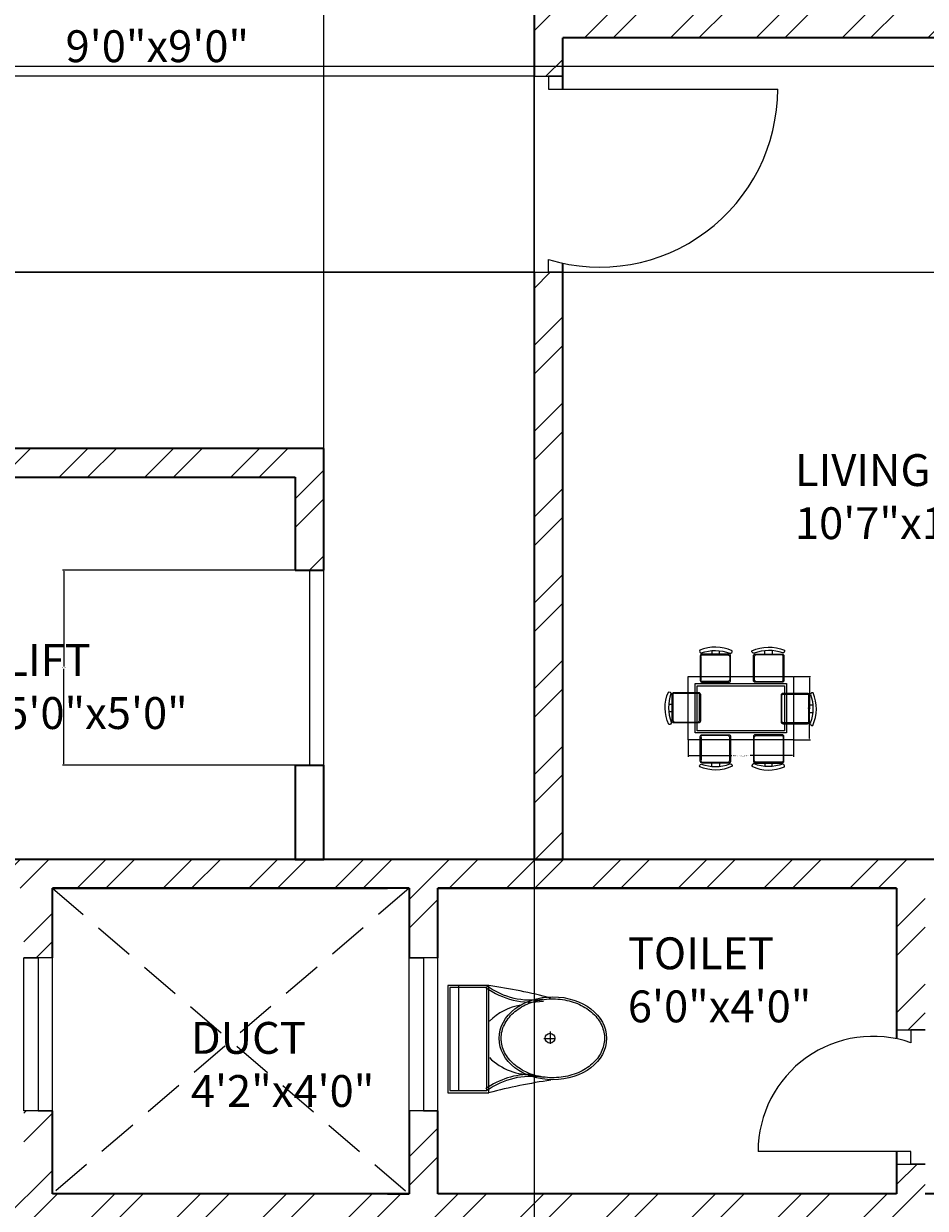
# Model space of a CAD drawing. Units: inches. Extents: x 1570 to 2186, y 1575 to 2421.
# Tile 4 of 10: x 1833 to 1975, y 1859 to 2045. Entities that reach past the tile are written whole.
import ezdxf

# ---------------------------------------------------------------- set-up
doc = ezdxf.new("R2010")
doc.units = ezdxf.units.IN
doc.linetypes.add('DASHED2', pattern=[9.525, 6.35, -3.175])
for name, color, linetype, lineweight in [('A-ANNO-DIMS', 2, 'Continuous', 18), ('A-AREA-IDEN', 7, 'Continuous', 18), ('A-DOOR', 201, 'Continuous', 18), ('A-FLOR-FIXT', 9, 'Continuous', 18), ('A-FLOR-OPEN', 254, 'DASHED2', 13), ('A-FURN', 8, 'Continuous', 13), ('A-GLAZ', 150, 'Continuous', 18), ('A-WALL', 7, 'Continuous', 35), ('A-WALL-PATT', 252, 'Continuous', 13)]:
    doc.layers.add(name, color=color, linetype=linetype, lineweight=lineweight)
doc.styles.get("Standard").update_dxf_attribs({"font": 'arial.ttf'})
doc.dimstyles.get("Standard").update_dxf_attribs({"dimtxt": 0.18, "dimasz": 0.18, "dimexe": 0.18, "dimexo": 0.0625, "dimgap": 0.09, "dimtad": 0, "dimtih": 1, "dimtoh": 1, "dimdec": 4, "dimzin": 0, "dimdsep": 46, "dimtxsty": 'Standard', "dimcen": 0.09, "dimadec": 0, "dimazin": 0, "dimtfac": 1, "dimtdec": 4, "dimtofl": 0, "dimtmove": 0, "dimatfit": 3, "dimfxl": 1, "dimtolj": 1, "dimtzin": 0, "dimarcsym": 0})

# ---------------------------------------------------------------- blocks, each defined once
blk = doc.blocks.new('A$C31115884')
for p, q in [((257.5, 466.4), (257.5, 523.2)), ((283.1, 497.7), (223.4, 497.7)), ((0, 200), (0, 0)), ((520, 200), (0, 200)), ((10, 190), (10, 10)), ((510, 190), (10, 190)), ((510, 10), (510, 190)), ((520, 0), (520, 200)), ((510, 54.5), (0, 54.5)), ((10, 10), (510, 10)), ((0, 0), (520, 0))]:
    blk.add_line(p, q)
blk.add_circle((255.6, 496.4), 23.6)
for centre, radius, start, end in [((2777.7, -204.6), 2807, 165.4549, 171.71327), ((-294.5, 403.3), 364.7, 324.20913, 9.34987), ((-294.5, 403.3), 374.7, 324.20913, 9.34987), ((805.8, 403.3), 364.7, 170.65013, 215.79087), ((3237, 905), 2807, 188.28673, 194.5451), ((139.5, 406.2), 293.5, 315.84364, 2.65635), ((805.8, 403.3), 374.7, 179.20365, 215.79087), ((383.6, 406.2), 293.5, 190.27735, 224.15636)]:
    blk.add_arc(centre, radius, start, end)
blk.add_ellipse((256.2, 509.9), major_axis=(0, -260.7), ratio=0.772727)
blk.add_open_spline([(256.2, 259.2), (263.1, 259.2), (270, 259.7), (287.8, 262.3), (298.7, 265.1), (319.9, 273.1), (330.2, 278.4), (350.1, 291.1), (359.7, 298.7), (377.7, 315.9), (386.2, 325.5), (401.7, 346.6), (408.8, 358.1), (421.3, 382.5), (426.8, 395.5), (435.9, 422.4), (439.5, 436.4), (444.8, 465.1), (446.5, 479.7), (447.9, 509.2), (447.6, 524), (445, 553.3), (442.7, 567.8), (436.3, 596), (432.1, 609.7), (421.9, 636), (416, 648.6), (402.5, 672.1), (395, 683), (378.6, 703), (369.8, 712.1), (351.1, 728), (341.3, 734.8), (320.9, 746.2), (310.4, 750.7), (288.9, 757.3), (278, 759.4), (256, 761), (245, 760.6), (223.1, 757.2), (212.3, 754.3), (191.1, 746.1), (180.8, 740.7), (160.9, 727.8), (151.4, 720.1), (133.5, 702.7), (125.1, 693), (109.6, 671.7), (102.6, 660.2), (90.2, 635.7), (84.9, 622.7), (76, 595.6), (72.4, 581.6), (67.2, 552.9), (65.6, 538.2), (64.4, 508.8), (64.8, 494), (67.5, 464.7), (69.9, 450.2), (76.6, 422), (80.8, 408.3), (91.1, 382.2), (97.2, 369.7), (110.8, 346.3), (118.4, 335.4), (134.8, 315.6), (143.7, 306.7), (162.4, 290.9), (172.3, 284.2), (192.8, 273), (203.3, 268.6), (224.8, 262.2), (235.8, 260.2), (249.9, 259.3), (253, 259.2), (256.2, 259.2)], degree=3, knots=[0, 0, 0, 0, 0.110105, 0.110105, 0.285049, 0.285049, 0.459994, 0.459994, 0.634938, 0.634938, 0.809882, 0.809882, 0.984827, 0.984827, 1.159771, 1.159771, 1.334715, 1.334715, 1.50966, 1.50966, 1.684604, 1.684604, 1.859549, 1.859549, 2.034493, 2.034493, 2.209437, 2.209437, 2.384382, 2.384382, 2.559326, 2.559326, 2.73427, 2.73427, 2.909215, 2.909215, 3.084159, 3.084159, 3.259103, 3.259103, 3.434048, 3.434048, 3.608992, 3.608992, 3.783936, 3.783936, 3.958881, 3.958881, 4.133825, 4.133825, 4.30877, 4.30877, 4.483714, 4.483714, 4.658658, 4.658658, 4.833603, 4.833603, 5.008547, 5.008547, 5.183491, 5.183491, 5.358436, 5.358436, 5.53338, 5.53338, 5.708324, 5.708324, 5.883269, 5.883269, 6.058213, 6.058213, 6.233158, 6.233158, 6.283185, 6.283185, 6.283185, 6.283185])
blk = doc.blocks.new('TABLE-DINING')
for points in [[(0, 9.93), (16.54, 9.93), (16.54, 0), (0, 0)], [(0, 9.93), (16.54, 9.93), (16.54, 0), (0, 0)], [(1.1, 8.82), (15.44, 8.82), (15.44, 1.1), (1.1, 1.1)], [(1.1, 8.82), (15.44, 8.82), (15.44, 1.1), (1.1, 1.1)], [(1.43, 8.49), (15.11, 8.49), (15.11, 1.43), (1.43, 1.43)], [(1.43, 8.49), (15.11, 8.49), (15.11, 1.43), (1.43, 1.43)]]:
    blk.add_lwpolyline(points, close=True)
blk = doc.blocks.new('WIN-24IN')
for p, q in [((2.25, 24), (0, 24)), ((0, 24), (4.5, 24)), ((0, 24), (0, 0)), ((2.25, 0), (2.25, 24)), ((4.5, 24), (4.5, 0)), ((0, 0), (4.5, 0)), ((4.5, 0), (2.25, 0))]:
    blk.add_line(p, q)
blk = doc.blocks.new('*D16')
at = {"layer": 'A-ANNO-DIMS', "color": 0, "lineweight": -2, "transparency": 16777216}
for p, q in [((1937.78, 1932.47), (1937.78, 1929.88)), ((1954.33, 1932.47), (1954.33, 1929.88)), ((1937.96, 1930.06), (1944.62, 1930.06)), ((1954.15, 1930.06), (1947.49, 1930.06))]:
    blk.add_line(p, q, dxfattribs=at)
at = {"layer": 'A-ANNO-DIMS', "color": 0, "transparency": 16777216}
for points in [[(1937.96, 1930.09), (1937.96, 1930.03), (1937.78, 1930.06)], [(1954.15, 1930.09), (1954.15, 1930.03), (1954.33, 1930.06)]]:
    blk.add_solid(points, dxfattribs=at)
at = {"layer": 'Defpoints', "color": 0, "transparency": 16777216}
for p in [(1937.78, 1932.54), (1954.33, 1932.54), (1954.33, 1930.06)]:
    blk.add_point(p, dxfattribs=at)
at = {"layer": 'A-ANNO-DIMS', "color": 0, "transparency": 16777216, "insert": (1946.06, 1930.06), "char_height": 0.18, "attachment_point": 5}
blk.add_mtext('\\A1;DINING TABLE 17 TYP.', dxfattribs=at)
blk = doc.blocks.new('*D17')
at = {"layer": 'A-ANNO-DIMS', "color": 0, "lineweight": -2, "transparency": 16777216}
for p, q in [((1954.39, 1942.46), (1956.99, 1942.46)), ((1956.81, 1942.28), (1956.81, 1937.68)), ((1956.81, 1932.72), (1956.81, 1937.32)), ((1954.39, 1932.54), (1956.99, 1932.54))]:
    blk.add_line(p, q, dxfattribs=at)
at = {"layer": 'A-ANNO-DIMS', "color": 0, "transparency": 16777216}
for points in [[(1956.78, 1942.28), (1956.84, 1942.28), (1956.81, 1942.46)], [(1956.78, 1932.72), (1956.84, 1932.72), (1956.81, 1932.54)]]:
    blk.add_solid(points, dxfattribs=at)
at = {"layer": 'Defpoints', "color": 0, "transparency": 16777216}
for p in [(1954.33, 1942.46), (1956.81, 1942.46), (1954.33, 1932.54)]:
    blk.add_point(p, dxfattribs=at)
at = {"layer": 'A-ANNO-DIMS', "color": 0, "transparency": 16777216, "insert": (1956.81, 1937.5), "char_height": 0.18, "attachment_point": 5}
blk.add_mtext('\\A1;10 TYP.', dxfattribs=at)
blk = doc.blocks.new('*D39')
at = {"layer": 'A-ANNO-DIMS', "color": 0, "lineweight": -2, "transparency": 16777216}
for p, q in [((1816.09, 2097.8), (1816.09, 1616.73)), ((1913.59, 2097.8), (1913.59, 1616.73)), ((1816.27, 1616.91), (1864.51, 1616.91)), ((1913.41, 1616.91), (1865.16, 1616.91))]:
    blk.add_line(p, q, dxfattribs=at)
at = {"layer": 'A-ANNO-DIMS', "color": 0, "transparency": 16777216}
for points in [[(1816.27, 1616.94), (1816.27, 1616.88), (1816.09, 1616.91)], [(1913.41, 1616.94), (1913.41, 1616.88), (1913.59, 1616.91)]]:
    blk.add_solid(points, dxfattribs=at)
at = {"layer": 'Defpoints', "color": 0, "transparency": 16777216}
for p in [(1816.09, 2097.86), (1913.59, 2097.86), (1913.59, 1616.91)]:
    blk.add_point(p, dxfattribs=at)
at = {"layer": 'A-ANNO-DIMS', "color": 0, "transparency": 16777216, "insert": (1864.84, 1616.91), "char_height": 0.18, "attachment_point": 5}
blk.add_mtext('\\A1;97.5', dxfattribs=at)
blk = doc.blocks.new('*D41')
at = {"layer": 'A-ANNO-DIMS', "color": 0, "lineweight": -2, "transparency": 16777216}
for p, q in [((1816.15, 2038.3), (2126.57, 2038.3)), ((2126.39, 2038.12), (2126.39, 2022.3)), ((2126.39, 2006.11), (2126.39, 2021.93)), ((1816.15, 2005.93), (2126.57, 2005.93))]:
    blk.add_line(p, q, dxfattribs=at)
at = {"layer": 'A-ANNO-DIMS', "color": 0, "transparency": 16777216}
for points in [[(2126.36, 2038.12), (2126.42, 2038.12), (2126.39, 2038.3)], [(2126.36, 2006.11), (2126.42, 2006.11), (2126.39, 2005.93)]]:
    blk.add_solid(points, dxfattribs=at)
at = {"layer": 'Defpoints', "color": 0, "transparency": 16777216}
for p in [(1816.09, 2038.3), (2126.39, 2038.3), (1816.09, 2005.93)]:
    blk.add_point(p, dxfattribs=at)
at = {"layer": 'A-ANNO-DIMS', "color": 0, "transparency": 16777216, "insert": (2126.39, 2022.12), "char_height": 0.18, "attachment_point": 5}
blk.add_mtext('\\A1;32.365', dxfattribs=at)
blk = doc.blocks.new('*D43')
at = {"layer": 'A-ANNO-DIMS', "color": 0, "lineweight": -2, "transparency": 16777216}
for p, q in [((1913.53, 2036.69), (1603.11, 2036.69)), ((1603.29, 2036.51), (1603.29, 2021.49)), ((1603.29, 2006.11), (1603.29, 2021.13)), ((1913.53, 2005.93), (1603.11, 2005.93))]:
    blk.add_line(p, q, dxfattribs=at)
at = {"layer": 'A-ANNO-DIMS', "color": 0, "transparency": 16777216}
for points in [[(1603.26, 2036.51), (1603.32, 2036.51), (1603.29, 2036.69)], [(1603.26, 2006.11), (1603.32, 2006.11), (1603.29, 2005.93)]]:
    blk.add_solid(points, dxfattribs=at)
at = {"layer": 'Defpoints', "color": 0, "transparency": 16777216}
for p in [(1603.29, 2036.69), (1913.59, 2036.69), (1913.59, 2005.93)]:
    blk.add_point(p, dxfattribs=at)
at = {"layer": 'A-ANNO-DIMS', "color": 0, "transparency": 16777216, "insert": (1603.29, 2021.31), "char_height": 0.18, "attachment_point": 5}
blk.add_mtext('\\A1;30.753', dxfattribs=at)
blk = doc.blocks.new('*D44')
at = {"layer": 'A-ANNO-DIMS', "color": 0, "lineweight": -2, "transparency": 16777216}
for p, q in [((1876.03, 1959.17), (1839.61, 1959.17)), ((1839.79, 1958.99), (1839.79, 1944.06)), ((1839.79, 1928.76), (1839.79, 1943.69)), ((1876.03, 1928.58), (1839.61, 1928.58))]:
    blk.add_line(p, q, dxfattribs=at)
at = {"layer": 'A-ANNO-DIMS', "color": 0, "transparency": 16777216}
for points in [[(1839.76, 1958.99), (1839.82, 1958.99), (1839.79, 1959.17)], [(1839.76, 1928.76), (1839.82, 1928.76), (1839.79, 1928.58)]]:
    blk.add_solid(points, dxfattribs=at)
at = {"layer": 'Defpoints', "color": 0, "transparency": 16777216}
for p in [(1839.79, 1959.17), (1876.09, 1959.17), (1876.09, 1928.58)]:
    blk.add_point(p, dxfattribs=at)
at = {"layer": 'A-ANNO-DIMS', "color": 0, "transparency": 16777216, "insert": (1839.79, 1943.88), "char_height": 0.18, "attachment_point": 5}
blk.add_mtext('\\A1;30.59', dxfattribs=at)
blk = doc.blocks.new('*D45')
at = {"layer": 'A-ANNO-DIMS', "color": 0, "lineweight": -2, "transparency": 16777216}
for p, q in [((1880.59, 1913.81), (1880.59, 2398.63)), ((1880.77, 2398.45), (1896.87, 2398.45)), ((1913.41, 2398.45), (1897.31, 2398.45)), ((1913.59, 1913.81), (1913.59, 2398.63))]:
    blk.add_line(p, q, dxfattribs=at)
at = {"layer": 'A-ANNO-DIMS', "color": 0, "transparency": 16777216}
for points in [[(1880.77, 2398.48), (1880.77, 2398.42), (1880.59, 2398.45)], [(1913.41, 2398.48), (1913.41, 2398.42), (1913.59, 2398.45)]]:
    blk.add_solid(points, dxfattribs=at)
at = {"layer": 'Defpoints', "color": 0, "transparency": 16777216}
for p in [(1913.59, 2398.45), (1880.59, 1913.75), (1913.59, 1913.75)]:
    blk.add_point(p, dxfattribs=at)
at = {"layer": 'A-ANNO-DIMS', "color": 0, "transparency": 16777216, "insert": (1897.09, 2398.45), "char_height": 0.18, "attachment_point": 5}
blk.add_mtext('\\A1;33', dxfattribs=at)

msp = doc.modelspace()

# ---------------------------------------------------------------- hatches: boundary and pattern name
at = {"layer": 'A-WALL-PATT'}
h = msp.add_hatch(dxfattribs=at)
h.set_pattern_fill('ANSI32', color=256)
h.paths.add_polyline_path([(1762.0975, 2362.1492), (1757.5975, 2362.1492), (1757.5975, 2357.6492), (1709.1163, 2357.6492), (1709.1163, 2362.1492), (1704.6163, 2362.1492), (1704.6163, 2353.1492), (1740.0886, 2353.1492), (1740.0886, 2261.8115), (1744.5886, 2261.8115), (1744.5886, 2353.1492), (1762.0975, 2353.1492)])
h.paths.add_polyline_path([(1890.2592, 2362.1492), (1885.7592, 2362.1492), (1826.5975, 2362.1492), (1822.0975, 2362.1492), (1822.0975, 2353.1492), (1862.5886, 2353.1492), (1862.5886, 2227.1492), (1744.5886, 2227.1492), (1744.5886, 2229.5389), (1742.3386, 2229.5389), (1740.0886, 2229.5389), (1740.0886, 2222.6492), (1744.5886, 2222.6492), (1756.186, 2222.6492), (1756.186, 2216.3571), (1760.686, 2216.3571), (1760.686, 2222.6492), (1832.686, 2222.6492), (1832.686, 2212.5994), (1837.186, 2212.5994), (1837.186, 2222.6492), (1893.186, 2222.6492), (1893.186, 2212.5994), (1897.686, 2212.5994), (1897.686, 2222.6492), (1989.5886, 2222.6492), (1989.5886, 2227.1492), (1989.5886, 2232.6585), (1987.3386, 2232.6585), (1985.0886, 2232.6585), (1985.0886, 2227.1492), (1867.0886, 2227.1492), (1867.0886, 2353.1492), (1890.2592, 2353.1492)])
h.paths.add_polyline_path([(1644.0886, 2353.1492), (1668.6163, 2353.1492), (1668.6163, 2362.1492), (1664.1163, 2362.1492), (1664.1163, 2358.9932), (1664.1163, 2357.6492), (1639.5886, 2357.6492), (1639.5886, 2213.8746), (1644.0886, 2213.8746), (1644.0886, 2222.6492), (1692.0886, 2222.6492), (1692.0886, 2215.9343), (1696.5886, 2215.9343), (1696.5886, 2222.6492), (1696.5886, 2227.1492), (1644.0886, 2227.1492)])
h.paths.add_polyline_path([(2013.0435, 2362.1492), (2008.5435, 2362.1492), (2008.5435, 2357.6492), (1954.7592, 2357.6492), (1954.7592, 2362.1492), (1950.2592, 2362.1492), (1950.2592, 2353.1492), (1985.0886, 2353.1492), (1985.0886, 2260.8534), (1989.5886, 2260.8534), (1989.5886, 2353.1492), (2013.0435, 2353.1492)])
h.paths.add_polyline_path([(2090.0886, 2357.6492), (2053.5435, 2357.6492), (2053.5435, 2362.1492), (2049.0435, 2362.1492), (2049.0435, 2353.1492), (2085.5886, 2353.1492), (2085.5886, 2227.1492), (2033.0886, 2227.1492), (2033.0886, 2222.6492), (2033.0886, 2214.4464), (2037.5886, 2214.4464), (2037.5886, 2222.6492), (2085.5886, 2222.6492), (2085.5886, 2212.4409), (2090.0886, 2212.4409)])
h.paths.add_polyline_path([(2090.0886, 2188.4409), (2087.8386, 2188.4409), (2085.5886, 2188.4409), (2085.5886, 2180.6492), (2037.5886, 2180.6492), (2037.5886, 2196.7956), (2033.0886, 2196.7956), (2033.0886, 2176.1492), (2037.5886, 2176.1492), (2045.0886, 2176.1492), (2045.0886, 2169.8988), (2049.5886, 2169.8988), (2049.5886, 2176.1492), (2085.5886, 2176.1492), (2085.5886, 2167.785), (2090.0886, 2167.785)])
h.paths.add_polyline_path([(2049.5886, 2147.4502), (2047.3386, 2147.4502), (2045.0886, 2147.4502), (2045.0886, 2124.4703), (2049.5886, 2124.4703)])
h.paths.add_polyline_path([(2090.0886, 2047.1492), (2049.5886, 2047.1492), (2049.5886, 2064.4703), (2045.0886, 2064.4703), (2045.0886, 2047.1492), (1918.0886, 2047.1492), (1918.0886, 2051.2061), (1913.5886, 2051.2061), (1913.5886, 2047.1492), (1913.5886, 2036.6872), (1918.0886, 2036.6872), (1918.0886, 2042.7492), (2045.0886, 2042.7492), (2045.0886, 2027.0686), (2049.5886, 2027.0686), (2049.5886, 2042.7492), (2090.0886, 2042.7492)])
h.paths.add_polyline_path([(1918.0886, 2005.9338), (1915.8386, 2005.9338), (1913.5886, 2005.9338), (1913.5886, 1913.7492), (1918.0886, 1913.7492)])
h.paths.add_polyline_path([(2090.0886, 1913.7492), (2049.5886, 1913.7492), (2045.0886, 1913.7492), (2033.0886, 1913.7492), (2033.0886, 1909.2492), (2033.0886, 1900.9803), (2037.5886, 1900.9803), (2037.5886, 1909.2492), (2085.5886, 1909.2492), (2085.5886, 1861.2492), (2037.5886, 1861.2492), (2037.5886, 1880.0859), (2033.0886, 1880.0859), (2033.0886, 1856.7492), (2085.5886, 1856.7492), (2085.5886, 1730.7492), (2054.2483, 1730.7492), (2054.2483, 1721.7492), (2058.7483, 1721.7492), (2058.7483, 1726.2492), (2090.0886, 1726.2492)])
h.paths.add_polyline_path([(2049.5886, 1967.0686), (2045.0886, 1967.0686), (2045.0886, 1913.7492), (2049.5886, 1913.7492)])
h.paths.add_polyline_path([(1989.5886, 1824.1695), (1987.3386, 1824.1695), (1985.0886, 1824.1695), (1985.0886, 1730.7492), (1989.5886, 1730.7492)])
h.paths.add_polyline_path([(1989.5886, 1861.2492), (1974.9963, 1861.2492), (1974.9963, 1865.9306), (1972.7463, 1865.9306), (1970.4963, 1865.9306), (1970.4963, 1861.2492), (1898.4963, 1861.2492), (1898.4963, 1874.2999), (1893.9963, 1874.2999), (1893.9963, 1861.2492), (1890.5886, 1861.2492), (1837.9963, 1861.2492), (1837.9963, 1874.3159), (1833.4963, 1874.3159), (1833.4963, 1861.2492), (1761.4963, 1861.2492), (1761.4963, 1865.0209), (1759.2463, 1865.0209), (1756.9963, 1865.0209), (1756.9963, 1861.2492), (1740.0886, 1861.2492), (1740.0886, 1856.7492), (1740.0886, 1850.7206), (1744.5886, 1850.7206), (1744.5886, 1856.7492), (1985.0886, 1856.7492), (1985.0886, 1851.0804), (1989.5886, 1851.0804), (1989.5886, 1856.7492)])
h.paths.add_polyline_path([(1989.5886, 1913.7492), (1740.0886, 1913.7492), (1740.0886, 1909.2492), (1756.9963, 1909.2492), (1756.9963, 1890.279), (1761.4963, 1890.279), (1761.4963, 1909.2492), (1833.4963, 1909.2492), (1833.4963, 1898.3159), (1837.9963, 1898.3159), (1837.9963, 1909.2492), (1890.5886, 1909.2492), (1893.9963, 1909.2492), (1893.9963, 1898.2999), (1898.4963, 1898.2999), (1898.4963, 1909.2492), (1970.4963, 1909.2492), (1970.4963, 1886.9887), (1974.9963, 1886.9887), (1974.9963, 1909.2492), (1989.5886, 1909.2492)])
h.paths.add_polyline_path([(1893.7344, 1730.7492), (1867.0886, 1730.7492), (1867.0886, 1856.7492), (1862.5886, 1856.7492), (1862.5886, 1730.7492), (1824.0492, 1730.7492), (1824.0492, 1721.7492), (1893.7344, 1721.7492)])
h.paths.add_polyline_path([(2018.2483, 1730.7492), (1953.7344, 1730.7492), (1953.7344, 1721.7492), (1958.2344, 1721.7492), (1958.2344, 1726.2492), (2013.7483, 1726.2492), (2013.7483, 1721.7492), (2018.2483, 1721.7492)])
h.paths.add_polyline_path([(1768.5492, 1730.7492), (1764.0492, 1730.7492), (1744.5886, 1730.7492), (1744.5886, 1819.4364), (1742.3386, 1819.4364), (1740.0886, 1819.4364), (1740.0886, 1730.7492), (1697.3801, 1730.7492), (1697.3801, 1721.7492), (1701.8801, 1721.7492), (1701.8801, 1726.2492), (1764.0492, 1726.2492), (1764.0492, 1721.7492), (1768.5492, 1721.7492)])
h.paths.add_polyline_path([(1644.0886, 1856.7492), (1639.5886, 1856.7492), (1639.5886, 1726.2492), (1657.0315, 1726.2492), (1657.0315, 1721.7492), (1661.3801, 1721.7492), (1661.3801, 1730.7492), (1644.0886, 1730.7492)])
h.paths.add_polyline_path([(1696.5886, 1876.1809), (1692.0886, 1876.1809), (1692.0886, 1861.2492), (1684.5886, 1861.2492), (1644.0886, 1861.2492), (1644.0886, 1909.2492), (1692.0886, 1909.2492), (1692.0886, 1900.3394), (1696.5886, 1900.3394), (1696.5886, 1913.7492), (1684.5886, 1913.7492), (1684.5886, 1920.2115), (1682.3386, 1920.2115), (1680.0886, 1920.2115), (1680.0886, 1913.7492), (1639.5886, 1913.7492), (1639.5886, 1856.7492), (1684.5886, 1856.7492), (1692.0886, 1856.7492), (1696.5886, 1856.7492)])
h.paths.add_polyline_path([(1684.5886, 2042.7492), (1811.5886, 2042.7492), (1811.5886, 2038.2991), (1816.0886, 2038.2991), (1816.0886, 2042.7492), (1816.0886, 2052.5708), (1813.8386, 2052.5708), (1811.5886, 2052.5708), (1811.5886, 2047.1492), (1684.5886, 2047.1492), (1684.5886, 2064.4703), (1680.0886, 2064.4703), (1680.0886, 2047.1492), (1639.5886, 2047.1492), (1639.5886, 2042.7492), (1680.0886, 2042.7492), (1680.0886, 2024.0762), (1684.5886, 2024.0762)])
h.paths.add_polyline_path([(1684.5886, 1964.0762), (1680.0886, 1964.0762), (1680.0886, 1944.6145), (1684.5886, 1944.6145)])
h.paths.add_polyline_path([(1816.0886, 1973.7492), (1876.0886, 1973.7492), (1876.0886, 1959.17), (1880.5886, 1959.17), (1880.5886, 1973.7492), (1880.5886, 1978.2492), (1816.0886, 1978.2492), (1816.0886, 2005.9338), (1813.8386, 2005.9338), (1811.5886, 2005.9338), (1811.5886, 1913.7492), (1816.0886, 1913.7492)])
h.paths.add_polyline_path([(1837.186, 2180.6492), (1837.186, 2188.5994), (1834.936, 2188.5994), (1832.686, 2188.5994), (1832.686, 2180.6492), (1760.686, 2180.6492), (1760.686, 2197.4807), (1756.186, 2197.4807), (1756.186, 2180.6492), (1744.5886, 2180.6492), (1740.0886, 2180.6492), (1740.0886, 2176.1492), (1837.186, 2176.1492)])
h.paths.add_polyline_path([(1974.186, 2196.8744), (1971.936, 2196.8744), (1969.686, 2196.8744), (1969.686, 2180.6492), (1897.686, 2180.6492), (1897.686, 2188.5994), (1895.436, 2188.5994), (1893.186, 2188.5994), (1893.186, 2180.6492), (1893.186, 2176.1492), (1974.186, 2176.1492)])
h.paths.add_polyline_path([(1918.0886, 2176.1492), (1913.5886, 2176.1492), (1913.5886, 2081.3709), (1918.0886, 2081.3709)])
h.paths.add_polyline_path([(1816.0886, 2176.1492), (1811.5886, 2176.1492), (1811.5886, 2081.3709), (1816.0886, 2081.3709)])
h.paths.add_polyline_path([(1684.5886, 2150.4939), (1682.3386, 2150.4939), (1680.0886, 2150.4939), (1680.0886, 2124.4703), (1684.5886, 2124.4703)])
h.paths.add_polyline_path([(1696.5886, 2180.6492), (1696.5886, 2197.4701), (1692.0886, 2197.4701), (1692.0886, 2180.6492), (1644.0886, 2180.6492), (1644.0886, 2189.8746), (1641.8386, 2189.8746), (1639.5886, 2189.8746), (1639.5886, 2169.814), (1644.0886, 2169.814), (1644.0886, 2176.1492), (1680.0886, 2176.1492), (1680.0886, 2171.7002), (1684.5886, 2171.7002), (1684.5886, 2176.1492), (1696.5886, 2176.1492)])

# ---------------------------------------------------------------- linework, layer by layer
at = {"layer": 'A-DOOR'}
for p, q in [((1913.5886, 2036.6872), (1918.0886, 2036.6872)), ((1918.0886, 2036.6872), (1915.8386, 2036.6872)), ((1915.8386, 2036.6872), (1915.8386, 2034.6872)), ((1915.8386, 2034.6872), (1951.8386, 2034.6872)), ((1915.8386, 2005.9338), (1915.8386, 2007.9338)), ((1913.5886, 2005.9338), (1918.0886, 2005.9338)), ((1918.0886, 2005.9338), (1915.8386, 2005.9338)), ((1878.3386, 1959.17), (1878.3386, 1928.5805)), ((1970.4963, 1886.9887), (1974.9963, 1886.9887)), ((1974.9963, 1886.9887), (1972.7463, 1886.9887)), ((1972.7463, 1886.9887), (1972.7463, 1884.9887)), ((1972.7463, 1867.9306), (1948.7463, 1867.9306)), ((1972.7463, 1865.9306), (1972.7463, 1867.9306)), ((1970.4963, 1865.9306), (1974.9963, 1865.9306)), ((1974.9963, 1865.9306), (1972.7463, 1865.9306))]:
    msp.add_line(p, q, dxfattribs=at)
for centre, radius, start, end in [((1923.8977, 2034.6872), 27.9409, 253.235828, 360), ((1966.8084, 1867.9306), 18.0621, 70.807153, 180)]:
    msp.add_arc(centre, radius, start, end, dxfattribs=at)
at = {"layer": 'A-FLOR-OPEN'}
for p, q in [((1893.9963, 1909.2492), (1837.9963, 1861.2492)), ((1837.9963, 1909.2492), (1893.9963, 1861.2492))]:
    msp.add_line(p, q, dxfattribs=at)
at = {"layer": 'A-FURN'}
for points in [[(1939.8309, 1946.1768, -0.17580919), (1944.3367, 1946.1427, 0.57839206), (1944.6781, 1946.5181, 0.21452438), (1939.592, 1946.5863, 0.55201397), (1939.8309, 1946.1768, -0.06507904)], [(1939.8309, 1946.1767, -0.17580919), (1944.3368, 1946.1426, 0.57839206), (1944.6781, 1946.5179, 0.21452438), (1939.592, 1946.5861, 0.55201397), (1939.8309, 1946.1767, -0.06507904)], [(1948.1301, 1946.1427, -0.57839206), (1947.7887, 1946.5181, -0.21452438), (1952.8748, 1946.5863, -0.55201397), (1952.6359, 1946.1768, 0.1758092), (1948.1301, 1946.1427)], [(1948.1301, 1946.1426, -0.57839206), (1947.7887, 1946.5179, -0.21452438), (1952.8749, 1946.5861, -0.55201397), (1952.6359, 1946.1767, 0.1758092), (1948.1301, 1946.1426)], [(1944.1456, 1945.996), (1939.9625, 1945.996, 0.41421356), (1939.6699, 1945.7034), (1939.6699, 1941.8571, 0.41421356), (1939.9625, 1941.5645), (1944.1456, 1941.5645, 0.41421356), (1944.4382, 1941.8571), (1944.4382, 1945.7034, 0.41421356), (1944.1456, 1945.996)], [(1944.1456, 1945.9958), (1939.9625, 1945.9958, 0.41421356), (1939.6699, 1945.7032), (1939.6699, 1941.8569, 0.41421356), (1939.9625, 1941.5643), (1944.1456, 1941.5643, 0.41421356), (1944.4382, 1941.8569), (1944.4382, 1945.7032, 0.41421356), (1944.1456, 1945.9958)], [(1942.6763, 1945.996), (1942.6763, 1946.525, -0.06475861)], [(1942.6763, 1945.9958), (1942.6763, 1946.5249, -0.06475861)], [(1952.5043, 1945.996, -0.41421356), (1952.7969, 1945.7034), (1952.7969, 1941.8571, -0.41421356), (1952.5043, 1941.5645), (1948.3212, 1941.5645, -0.41421356), (1948.0286, 1941.8571), (1948.0286, 1945.7034, -0.41421356), (1948.3212, 1945.996), (1952.5043, 1945.996)], [(1952.5043, 1945.9958, -0.41421356), (1952.7969, 1945.7032), (1952.7969, 1941.8569, -0.41421356), (1952.5043, 1941.5643), (1948.3212, 1941.5643, -0.41421356), (1948.0286, 1941.8569), (1948.0286, 1945.7032, -0.41421356), (1948.3212, 1945.9958), (1952.5043, 1945.9958)], [(1949.7905, 1945.996), (1949.7905, 1946.525, 0.06475861)], [(1949.7905, 1945.9958), (1949.7905, 1946.5249, 0.06475861)], [(1935.117, 1935.296, -0.57839206), (1934.7416, 1934.9546, -0.21452438), (1934.6734, 1940.0407, -0.55201397), (1935.0828, 1939.8018, 0.17580937), (1935.117, 1935.296)], [(1935.117, 1935.2958, -0.57839206), (1934.7416, 1934.9544, -0.21452438), (1934.6734, 1940.0406, -0.55201397), (1935.0829, 1939.8016, 0.17580937), (1935.117, 1935.2958)], [(1935.2637, 1939.6702, -0.41421356), (1935.5563, 1939.9628), (1939.4026, 1939.9628, -0.41421356), (1939.6952, 1939.6702), (1939.6952, 1935.4871, -0.41421356), (1939.4026, 1935.1945), (1935.5563, 1935.1945, -0.41421356), (1935.2637, 1935.4871), (1935.2637, 1939.6702)], [(1935.2637, 1939.67, -0.41421356), (1935.5563, 1939.9627), (1939.4026, 1939.9627, -0.41421356), (1939.6952, 1939.67), (1939.6952, 1935.487, -0.41421356), (1939.4026, 1935.1943), (1935.5563, 1935.1943, -0.41421356), (1935.2637, 1935.487), (1935.2637, 1939.67)], [(1956.8045, 1939.5269, 0.41421356), (1956.5118, 1939.8196), (1952.6656, 1939.8196, 0.41421356), (1952.3729, 1939.5269), (1952.3729, 1935.3439, 0.41421356), (1952.6656, 1935.0512), (1956.5118, 1935.0512, 0.41421356), (1956.8045, 1935.3439), (1956.8045, 1939.5269)], [(1956.8045, 1939.5267, 0.41421356), (1956.5118, 1939.8194), (1952.6656, 1939.8194, 0.41421356), (1952.3729, 1939.5267), (1952.3729, 1935.3437, 0.41421356), (1952.6656, 1935.051), (1956.5118, 1935.051, 0.41421356), (1956.8045, 1935.3437), (1956.8045, 1939.5267)], [(1956.9853, 1939.6585, -0.17580919), (1956.9512, 1935.1527, 0.57839206), (1957.3265, 1934.8114, 0.21452438), (1957.3948, 1939.8975, 0.55201397), (1956.9853, 1939.6585, -0.06507904)], [(1956.9853, 1939.6584, -0.17580919), (1956.9512, 1935.1525, 0.57839206), (1957.3265, 1934.8112, 0.21452438), (1957.3948, 1939.8973, 0.55201397), (1956.9853, 1939.6584, -0.06507904)], [(1935.2637, 1936.9564), (1934.7347, 1936.9564, 0.06475861)], [(1935.2637, 1936.9563), (1934.7347, 1936.9563, 0.06475861)], [(1956.8045, 1936.8132), (1957.3335, 1936.8132, -0.06475861)], [(1956.8045, 1936.813), (1957.3335, 1936.813, -0.06475861)], [(1944.1456, 1928.8985), (1939.9625, 1928.8985, -0.41421356), (1939.6699, 1929.1912), (1939.6699, 1933.0374, -0.41421356), (1939.9625, 1933.3301), (1944.1456, 1933.3301, -0.41421356), (1944.4382, 1933.0374), (1944.4382, 1929.1912, -0.41421356), (1944.1456, 1928.8985)], [(1944.1456, 1928.8984), (1939.9625, 1928.8984, -0.41421356), (1939.6699, 1929.191), (1939.6699, 1933.0372, -0.41421356), (1939.9625, 1933.3299), (1944.1456, 1933.3299, -0.41421356), (1944.4382, 1933.0372), (1944.4382, 1929.191, -0.41421356), (1944.1456, 1928.8984)], [(1952.5043, 1928.8985, 0.41421356), (1952.7969, 1929.1912), (1952.7969, 1933.0374, 0.41421356), (1952.5043, 1933.3301), (1948.3212, 1933.3301, 0.41421356), (1948.0286, 1933.0374), (1948.0286, 1929.1912, 0.41421356), (1948.3212, 1928.8985), (1952.5043, 1928.8985)], [(1952.5043, 1928.8984, 0.41421356), (1952.7969, 1929.191), (1952.7969, 1933.0372, 0.41421356), (1952.5043, 1933.3299), (1948.3212, 1933.3299, 0.41421356), (1948.0286, 1933.0372), (1948.0286, 1929.191, 0.41421356), (1948.3212, 1928.8984), (1952.5043, 1928.8984)], [(1944.3367, 1928.7518, -0.57839206), (1944.6781, 1928.3765, -0.21452438), (1939.592, 1928.3082, -0.55201397), (1939.8309, 1928.7177, 0.17580929), (1944.3367, 1928.7518)], [(1944.3368, 1928.7516, -0.57839206), (1944.6781, 1928.3763, -0.21452438), (1939.592, 1928.308, -0.55201397), (1939.8309, 1928.7175, 0.17580929), (1944.3368, 1928.7516)], [(1942.6763, 1928.8985), (1942.6763, 1928.3695, 0.06475861)], [(1942.6763, 1928.8984), (1942.6763, 1928.3693, 0.06475861)], [(1952.6359, 1928.7177, -0.17580928), (1948.1301, 1928.7518, 0.57839206), (1947.7887, 1928.3765, 0.21452438), (1952.8748, 1928.3082, 0.55201397), (1952.6359, 1928.7177, -0.06507904)], [(1952.6359, 1928.7175, -0.17580928), (1948.1301, 1928.7516, 0.57839206), (1947.7887, 1928.3763, 0.21452438), (1952.8749, 1928.308, 0.55201397), (1952.6359, 1928.7175, -0.06507904)], [(1949.7905, 1928.8985), (1949.7905, 1928.3695, -0.06475861)], [(1949.7905, 1928.8984), (1949.7905, 1928.3693, -0.06475861)]]:
    msp.add_lwpolyline(points, format="xyb", dxfattribs=at)
for points in [[(1939.9643, 1945.8642), (1944.0137, 1945.8642, -0.41421356), (1944.3064, 1945.5715), (1944.3064, 1941.989, -0.41421356), (1944.0137, 1941.6963), (1939.9643, 1941.6963, -0.51206948), (1939.8017, 1941.989), (1939.8017, 1945.5715, -0.51206948)], [(1939.9643, 1945.864), (1944.0138, 1945.864, -0.41421356), (1944.3064, 1945.5713), (1944.3064, 1941.9888, -0.41421356), (1944.0138, 1941.6961), (1939.9643, 1941.6961, -0.51206948), (1939.8017, 1941.9888), (1939.8017, 1945.5713, -0.51206948)], [(1952.5025, 1945.8642), (1948.4531, 1945.8642, 0.41421356), (1948.1604, 1945.5715), (1948.1604, 1941.989, 0.41421356), (1948.4531, 1941.6963), (1952.5025, 1941.6963, 0.51206948), (1952.6651, 1941.989), (1952.6651, 1945.5715, 0.51206948)], [(1952.5025, 1945.864), (1948.4531, 1945.864, 0.41421356), (1948.1604, 1945.5713), (1948.1604, 1941.9888, 0.41421356), (1948.4531, 1941.6961), (1952.5025, 1941.6961, 0.51206948), (1952.6651, 1941.9888), (1952.6651, 1945.5713, 0.51206948)], [(1935.3955, 1939.6684), (1935.3955, 1935.619, 0.41421356), (1935.6882, 1935.3263), (1939.2707, 1935.3263, 0.41421356), (1939.5634, 1935.619), (1939.5634, 1939.6684, 0.51206948), (1939.2707, 1939.831), (1935.6882, 1939.831, 0.51206948)], [(1935.3955, 1939.6682), (1935.3955, 1935.6188, 0.41421356), (1935.6882, 1935.3261), (1939.2707, 1935.3261, 0.41421356), (1939.5634, 1935.6188), (1939.5634, 1939.6682, 0.51206948), (1939.2707, 1939.8308), (1935.6882, 1939.8308, 0.51206948)], [(1956.6726, 1939.5251), (1956.6726, 1935.4757, -0.41421356), (1956.38, 1935.1831), (1952.7974, 1935.1831, -0.41421356), (1952.5048, 1935.4757), (1952.5048, 1939.5251, -0.51206948), (1952.7974, 1939.6877), (1956.38, 1939.6877, -0.51206948)], [(1956.6726, 1939.525), (1956.6726, 1935.4755, -0.41421356), (1956.38, 1935.1829), (1952.7974, 1935.1829, -0.41421356), (1952.5048, 1935.4755), (1952.5048, 1939.525, -0.51206948), (1952.7974, 1939.6876), (1956.38, 1939.6876, -0.51206948)], [(1939.9643, 1929.0304), (1944.0137, 1929.0304, 0.41421356), (1944.3064, 1929.323), (1944.3064, 1932.9056, 0.41421356), (1944.0137, 1933.1982), (1939.9643, 1933.1982, 0.51206948), (1939.8017, 1932.9056), (1939.8017, 1929.323, 0.51206948)], [(1939.9643, 1929.0302), (1944.0138, 1929.0302, 0.41421356), (1944.3064, 1929.3228), (1944.3064, 1932.9054, 0.41421356), (1944.0138, 1933.1981), (1939.9643, 1933.1981, 0.51206948), (1939.8017, 1932.9054), (1939.8017, 1929.3228, 0.51206948)], [(1952.5025, 1929.0304), (1948.4531, 1929.0304, -0.41421356), (1948.1604, 1929.323), (1948.1604, 1932.9056, -0.41421356), (1948.4531, 1933.1982), (1952.5025, 1933.1982, -0.51206948), (1952.6651, 1932.9056), (1952.6651, 1929.323, -0.51206948)], [(1952.5025, 1929.0302), (1948.4531, 1929.0302, -0.41421356), (1948.1604, 1929.3228), (1948.1604, 1932.9054, -0.41421356), (1948.4531, 1933.1981), (1952.5025, 1933.1981, -0.51206948), (1952.6651, 1932.9054), (1952.6651, 1929.3228, -0.51206948)]]:
    msp.add_lwpolyline(points, format="xyb", close=True, dxfattribs=at)
for points in [[(1941.5054, 1946.5346), (1941.5054, 1945.996)], [(1941.5054, 1946.5345), (1941.5054, 1945.9958)], [(1950.9614, 1946.5346), (1950.9614, 1945.996)], [(1950.9614, 1946.5345), (1950.9614, 1945.9958)], [(1934.725, 1938.1273), (1935.2637, 1938.1273)], [(1934.7251, 1938.1272), (1935.2637, 1938.1272)], [(1957.3431, 1937.9841), (1956.8045, 1937.9841)], [(1957.3431, 1937.9839), (1956.8045, 1937.9839)], [(1941.5054, 1928.3599), (1941.5054, 1928.8985)], [(1941.5054, 1928.3597), (1941.5054, 1928.8984)], [(1950.9614, 1928.3599), (1950.9614, 1928.8985)], [(1950.9614, 1928.3597), (1950.9614, 1928.8984)]]:
    msp.add_lwpolyline(points, dxfattribs=at)
at = {"layer": 'A-WALL'}
for p, q in [((1913.5886, 2047.1492), (1913.5886, 2036.6872)), ((2045.0886, 2042.7492), (1918.0886, 2042.7492)), ((1918.0886, 2034.6872), (1918.0886, 2042.7492)), ((1918.0886, 1913.7492), (1918.0886, 2007.3569)), ((1913.5886, 2005.9338), (1913.5886, 1913.7492)), ((1880.5886, 1978.2492), (1816.0886, 1978.2492)), ((1880.5886, 1973.7492), (1880.5886, 1978.2492)), ((1816.0886, 1973.7492), (1876.0886, 1973.7492)), ((1876.0886, 1973.7492), (1876.0886, 1959.17)), ((1880.5886, 1959.17), (1880.5886, 1973.7492)), ((1876.0886, 1959.17), (1880.5886, 1959.17)), ((1876.0886, 1928.5805), (1880.5886, 1928.5805)), ((1876.0886, 1928.5805), (1876.0886, 1913.7492)), ((1880.5886, 1913.7492), (1880.5886, 1928.5805)), ((1989.5886, 1913.7492), (1740.0886, 1913.7492)), ((1876.0886, 1913.7492), (1880.5886, 1913.7492)), ((1913.5886, 1913.7492), (1918.0886, 1913.7492)), ((1837.9963, 1909.2492), (1890.5886, 1909.2492)), ((1837.9963, 1898.3159), (1837.9963, 1909.2492)), ((1893.9963, 1909.2492), (1837.9963, 1909.2492)), ((1893.9963, 1909.2492), (1893.9963, 1898.2999)), ((1898.4963, 1909.2492), (1970.4963, 1909.2492)), ((1898.4963, 1898.2999), (1898.4963, 1909.2492)), ((1970.4963, 1909.2492), (1898.4963, 1909.2492)), ((1970.4963, 1909.2492), (1970.4963, 1885.6122)), ((1837.9963, 1861.2492), (1837.9963, 1874.3159)), ((1893.9963, 1874.2999), (1893.9963, 1861.2492)), ((1898.4963, 1861.2492), (1898.4963, 1874.2999)), ((1970.4963, 1867.9306), (1970.4963, 1861.2492)), ((1893.9963, 1861.2492), (1837.9963, 1861.2492)), ((1890.5886, 1861.2492), (1893.9963, 1861.2492)), ((1970.4963, 1861.2492), (1898.4963, 1861.2492)), ((1989.5886, 1861.2492), (1974.9963, 1861.2492))]:
    msp.add_line(p, q, dxfattribs=at)

# ---------------------------------------------------------------- block references
at = {"layer": 'A-FLOR-FIXT', "xscale": 0.0323450304620732, "yscale": 0.0323450304620732, "zscale": 0.0323450304620732, "rotation": 269.9999999999999}
msp.add_blockref('A$C31115884', (1900.0497, 1893.9691), dxfattribs=at)
at = {"layer": 'A-FURN'}
msp.add_blockref('TABLE-DINING', (1937.7843, 1932.5374), dxfattribs=at)
at = {"layer": 'A-GLAZ', "rotation": 180}
for p in [(1837.996, 1898.3158), (1898.496, 1898.2998)]:
    msp.add_blockref('WIN-24IN', p, dxfattribs=at)

# ---------------------------------------------------------------- texts
at = {"layer": 'A-AREA-IDEN', "char_height": 5, "attachment_point": 1}
for s, width, insert in [('LOBBY\\P9\'0"x9\'0"', 115.828202, (1840.0646, 2052.2484)), ('LIVING\\P10\'7"x10\'9"', 144.692974, (1954.5434, 1977.3775)), ('LIFT\\P5\'0"x5\'0"', 119.411331, (1830.4398, 1947.5705)), ('TOILET\\P6\'0"x4\'0"', 104.586025, (1928.3144, 1901.5278)), ('DUCT\\P4\'2"x4\'0"', 79.322095, (1859.7287, 1888.2483))]:
    msp.add_mtext_dynamic_manual_height_columns(s, width=width, gutter_width=12.5, heights=[0], dxfattribs=dict(at, insert=insert))

# ---------------------------------------------------------------- dimensions: what is measured, and where the dimension line sits
at = {"layer": 'A-ANNO-DIMS'}
for base, p1, p2, override, picture, middle in [((1913.5886, 2398.4492), (1880.5886, 1913.7492), (1913.5886, 1913.7492), {"dimdec": 0, "dimlfac": 1, "dimrnd": 0, "dimzin": 0, "dimdsep": 46, "dimlunit": 2}, '*D45', (1897.0886, 2398.4492)), ((1913.5886, 1616.9104), (1816.0886, 2097.8597), (1913.5886, 2097.8597), {"dimdec": 1, "dimlfac": 1, "dimrnd": 0, "dimzin": 0, "dimdsep": 46, "dimlunit": 2}, '*D39', (1864.8386, 1616.9104))]:
    dim = msp.add_linear_dim(base=base, p1=p1, p2=p2, dimstyle='Standard', override=override, dxfattribs=at)
    dim.commit()
    dim.dimension.update_dxf_attribs({"geometry": picture, "text_midpoint": middle})
for base, p1, p2, override, picture, middle in [((2126.3886, 2038.2991), (1816.0886, 2005.9338), (1816.0886, 2038.2991), {"dimdec": 3, "dimlfac": 1, "dimrnd": 0, "dimzin": 0, "dimdsep": 46, "dimlunit": 2}, '*D41', (2126.3886, 2022.1164)), ((1603.2886, 2036.6872), (1913.5886, 2005.9338), (1913.5886, 2036.6872), {"dimdec": 3, "dimlfac": 1, "dimrnd": 0, "dimzin": 0, "dimdsep": 46, "dimlunit": 2}, '*D43', (1603.2886, 2021.3105)), ((1839.7886, 1959.17), (1876.0886, 1928.5805), (1876.0886, 1959.17), {"dimdec": 2, "dimlfac": 1, "dimrnd": 0, "dimzin": 0, "dimdsep": 46, "dimlunit": 2}, '*D44', (1839.7886, 1943.8752))]:
    dim = msp.add_linear_dim(base=base, p1=p1, p2=p2, angle=90, dimstyle='Standard', override=override, dxfattribs=at)
    dim.commit()
    dim.dimension.update_dxf_attribs({"geometry": picture, "text_midpoint": middle})
dim = msp.add_linear_dim(base=(1956.8091, 1942.4633), p1=(1954.3277, 1932.5374), p2=(1954.3277, 1942.4633), angle=90, text='<> TYP.', dimstyle='Standard', override={"dimdec": 0, "dimlfac": 1, "dimrnd": 0, "dimzin": 0, "dimdsep": 46, "dimlunit": 2}, dxfattribs=at)
dim.commit()
dim.dimension.update_dxf_attribs({"geometry": '*D17', "text_midpoint": (1956.8091, 1937.5003)})
dim = msp.add_linear_dim(base=(1954.3277, 1930.0559), p1=(1937.7847, 1932.5374), p2=(1954.3277, 1932.5374), text='DINING TABLE <> TYP.', dimstyle='Standard', override={"dimdec": 0, "dimlfac": 1, "dimrnd": 0, "dimzin": 0, "dimdsep": 46, "dimlunit": 2}, dxfattribs=at)
dim.commit()
dim.dimension.update_dxf_attribs({"geometry": '*D16', "text_midpoint": (1946.0562, 1930.0559)})

doc.saveas('drawing.dxf')
